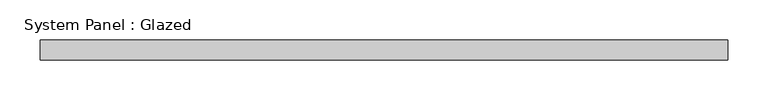
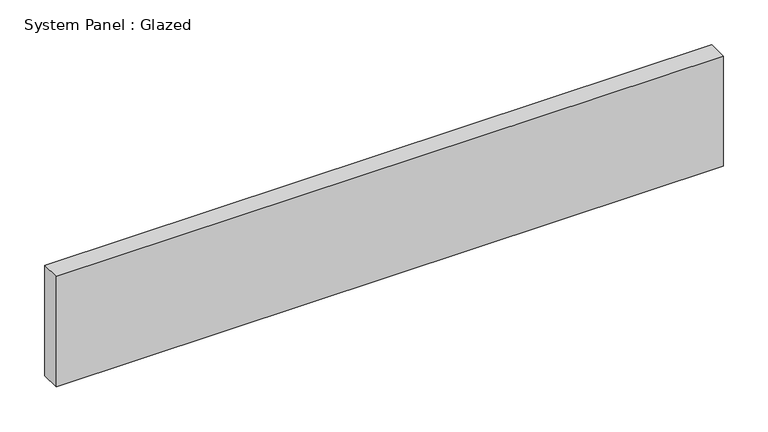
"""IFC4 building model written with IfcOpenShell, lengths in millimetres: plate geometry, System Panel : Glazed."""

from ifc_helpers import new_model, si_unit, origin, origin_with_axes, place, context, project, spatial, polyline, outline, extrude, source, transform, mapped, element, save


def system_panel_glazed_747750e0(model_context):
    return source(origin(), model_context, "Body", "SweptSolid", [
        extrude(outline(polyline([(428.9578978, 24.5), (-428.9578978, 24.5), (-428.9578978, 49.5), (428.9578978, 49.5), (428.9578978, 24.5)])), origin_with_axes(), (0.0, 0.0, 1.0), 150.0429688),
    ])


if __name__ == "__main__":
    model = new_model("IFC4")
    model_context = context("Model", 3, world=origin())
    ifc_project = project(units=[si_unit("LENGTHUNIT", "METRE", prefix="MILLI")], contexts=[model_context])
    site = spatial("IfcSite", under=ifc_project)
    building = spatial("IfcBuilding", under=site)
    placement = place(None, origin())
    system_panel_glazed_shape = system_panel_glazed_747750e0(model_context)
    element("IfcPlate", 1, ObjectType="System Panel : Glazed", at=placement, inside=building, context=model_context, shape_type="MappedRepresentation", body=[
        mapped(system_panel_glazed_shape, transform((0.0, 0.0, 0.0), x_axis=(1.0, 0.0, 0.0), y_axis=(0.0, 1.0, 0.0), z_axis=(0.0, 0.0, 1.0))),
    ])
    save(model, "model.ifc")

# Revit data of these elements
# Type "System Panel : Glazed"
#   Keynote = "H11"
#   Construction Type Id = "GSP4R"
#   Analytic Construction = "1/8 in Pilkington single glazing"
#   Visual Light Transmittance = 0.9
#   Solar Heat Gain Coefficient = 0.86
#   Heat Transfer Coefficient (U) = 6.7069 W/(m²·K)
#   Define Thermal Properties by = 1
# Element 1 (IfcPlate, "System Panel : Glazed")
#   Materials on its faces: "Glass"
# Materials
#   "Glass": class "Glass", colour RGB 0 128 192, transparency 0.9, Description = "Soda Lime Glass", Cost = 0
